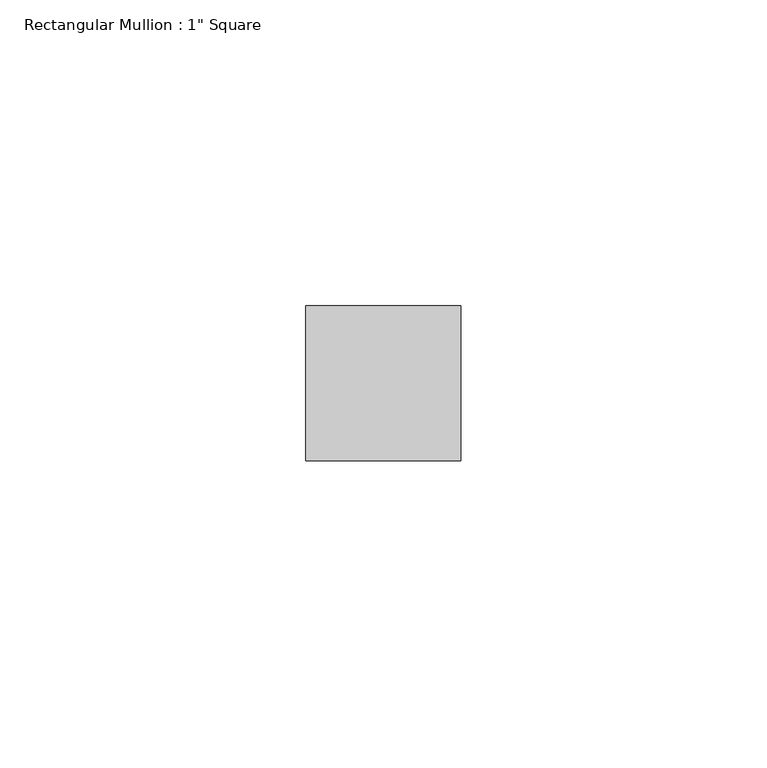
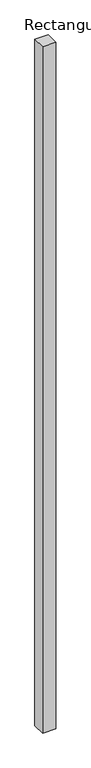
"""IFC4 building model written with IfcOpenShell, lengths in millimetres: member geometry."""

from ifc_helpers import new_model, si_unit, frame, origin, place, context, project, spatial, polyline, outline, extrude, source, transform, mapped, element, save


def member_dc2600c8(model_context):
    return source(origin(), model_context, "Body", "SweptSolid", [
        extrude(outline(polyline([(12.7, 12.7), (12.7, -12.7), (-12.7, -12.7), (-12.7, 12.7), (12.7, 12.7)])), frame((0.0, 0.0, -1397.0), z_axis=(0.0, 0.0, 1.0), x_axis=(1.0, 0.0, 0.0)), (0.0, 0.0, 1.0), 1397.0),
    ])


if __name__ == "__main__":
    model = new_model("IFC4")
    model_context = context("Model", 3, world=origin())
    ifc_project = project(units=[si_unit("LENGTHUNIT", "METRE", prefix="MILLI")], contexts=[model_context])
    site = spatial("IfcSite", under=ifc_project)
    building = spatial("IfcBuilding", under=site)
    placement = place(None, origin())
    member_shape = member_dc2600c8(model_context)
    element("IfcMember", 1, ObjectType="Rectangular Mullion : 1\" Square", at=placement, inside=building, context=model_context, shape_type="MappedRepresentation", body=[
        mapped(member_shape, transform((0.0, 0.0, 0.0), x_axis=(1.0, 0.0, 0.0), y_axis=(0.0, 1.0, 0.0), z_axis=(0.0, 0.0, 1.0))),
    ])
    save(model, "model.ifc")

# Revit data of these elements
# Type "Rectangular Mullion : 1\" Square"
#   built-in parameter 1007304 = 0.0833333 (stored number, unit not read)
#   built-in parameter 1007301 = 0.0416667 (stored number, unit not read)
#   built-in parameter 1007300 = 0.0416667 (stored number, unit not read)
